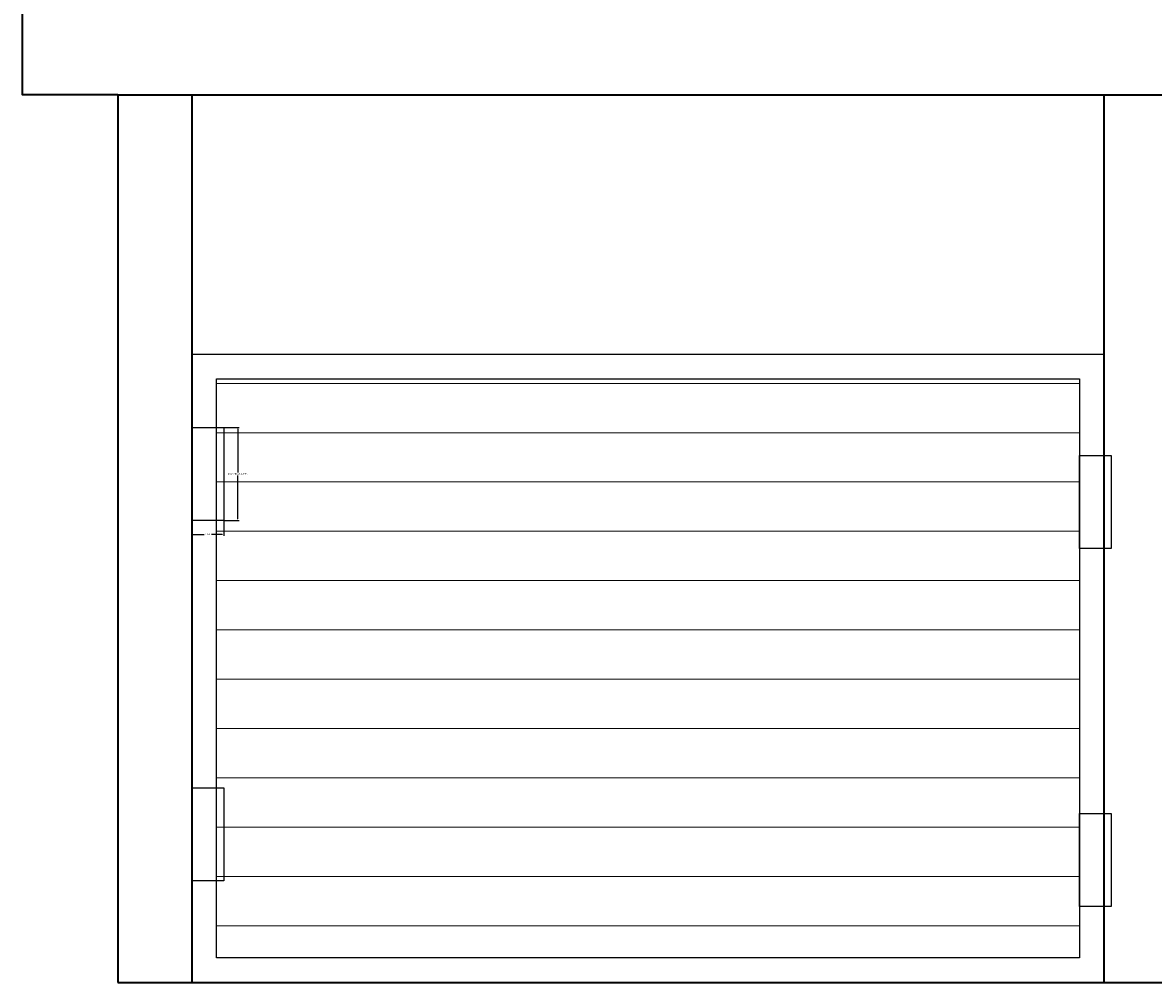
# Model space of a CAD drawing. Units: inches. Extents: x 3 to 303, y 4 to 326.
# Tile 1 of 6: x 4 to 141, y 4 to 120. Entities that reach past the tile are written whole.
import ezdxf

# ---------------------------------------------------------------- set-up
doc = ezdxf.new("R2010")
doc.units = ezdxf.units.IN
doc.header["$MEASUREMENT"] = 0
for name, color, linetype, lineweight in [('A-ANNO-DIMS', 2, 'Continuous', 18), ('A-DOOR', 3, 'Continuous', 25), ('A-ELEV', 7, 'Continuous', 35), ('A-ELEV-PATT', 8, 'Continuous', 13)]:
    doc.layers.add(name, color=color, linetype=linetype, lineweight=lineweight)
doc.styles.get("Standard").update_dxf_attribs({"font": 'arial.ttf'})
doc.dimstyles.get("Standard").update_dxf_attribs({"dimtxt": 0.18, "dimasz": 0.18, "dimexe": 0.18, "dimexo": 0.0625, "dimgap": 0.09, "dimtad": 0, "dimtih": 1, "dimtoh": 1, "dimdec": 4, "dimzin": 0, "dimdsep": 46, "dimtxsty": 'Standard', "dimcen": 0.09, "dimadec": 0, "dimazin": 0, "dimtfac": 1, "dimtdec": 4, "dimtofl": 0, "dimtmove": 0, "dimatfit": 3, "dimfxl": 1, "dimtolj": 1, "dimtzin": 0, "dimarcsym": 0})

# ---------------------------------------------------------------- blocks, each defined once
blk = doc.blocks.new('HINGE')
blk.add_lwpolyline([(171.8, 207.5), (175.68, 207.5), (175.68, 196.19), (171.8, 196.19)], close=True)
blk = doc.blocks.new('*D6')
at = {"layer": 'A-ANNO-DIMS', "color": 0, "lineweight": -2, "transparency": 16777216}
for p, q in [((28.18, 71.14), (29.99, 71.14)), ((29.81, 70.96), (29.81, 65.67)), ((29.81, 60.01), (29.81, 65.3)), ((28.18, 59.83), (29.99, 59.83))]:
    blk.add_line(p, q, dxfattribs=at)
at = {"layer": 'A-ANNO-DIMS', "color": 0, "transparency": 16777216}
for points in [[(29.78, 70.96), (29.84, 70.96), (29.81, 71.14)], [(29.78, 60.01), (29.84, 60.01), (29.81, 59.83)]]:
    blk.add_solid(points, dxfattribs=at)
at = {"layer": 'Defpoints', "color": 0, "transparency": 16777216}
for p in [(28.11, 71.14), (29.81, 71.14), (28.11, 59.83)]:
    blk.add_point(p, dxfattribs=at)
at = {"layer": 'A-ANNO-DIMS', "color": 0, "transparency": 16777216, "insert": (29.81, 65.49), "char_height": 0.18, "attachment_point": 5}
blk.add_mtext('\\A1;DOOR HINGE 11 TYP.', dxfattribs=at)
blk = doc.blocks.new('*D7')
at = {"layer": 'A-ANNO-DIMS', "color": 0, "lineweight": -2, "transparency": 16777216}
for p, q in [((24.23, 59.77), (24.23, 57.95)), ((28.11, 59.77), (28.11, 57.95)), ((24.41, 58.13), (25.71, 58.13)), ((27.93, 58.13), (26.63, 58.13))]:
    blk.add_line(p, q, dxfattribs=at)
at = {"layer": 'A-ANNO-DIMS', "color": 0, "transparency": 16777216}
for points in [[(24.41, 58.16), (24.41, 58.1), (24.23, 58.13)], [(27.93, 58.16), (27.93, 58.1), (28.11, 58.13)]]:
    blk.add_solid(points, dxfattribs=at)
at = {"layer": 'Defpoints', "color": 0, "transparency": 16777216}
for p in [(24.23, 59.83), (28.11, 59.83), (28.11, 58.13)]:
    blk.add_point(p, dxfattribs=at)
at = {"layer": 'A-ANNO-DIMS', "color": 0, "transparency": 16777216, "insert": (26.17, 58.13), "char_height": 0.18, "attachment_point": 5}
blk.add_mtext('\\A1;4 TYP.', dxfattribs=at)

msp = doc.modelspace()

# ---------------------------------------------------------------- hatches: boundary and pattern name
at = {"layer": 'A-ELEV-PATT'}
h = msp.add_hatch(dxfattribs=at)
h.set_pattern_fill('_USER', color=256, scale=6, pattern_type=0)
h.set_pattern_definition([(0, (-9.712, -25.502), (0, 6), [])])
h.paths.add_polyline_path([(132.23, 77.06), (27.23, 77.06), (27.23, 6.62), (132.23, 6.62)])

# ---------------------------------------------------------------- linework, layer by layer
at = {"layer": 'A-DOOR'}
for points in [[(24.23, 80.06), (135.23, 80.06), (135.23, 3.62), (24.23, 3.62)], [(27.23, 77.06), (132.23, 77.06), (132.23, 6.62), (27.23, 6.62)]]:
    msp.add_lwpolyline(points, close=True, dxfattribs=at)
at = {"layer": 'A-ELEV'}
for p, q in [((15.23, 111.62), (15.23, 3.62)), ((15.23, 111.62), (219.23, 111.62)), ((24.23, 111.62), (24.23, 3.62)), ((135.23, 3.62), (135.23, 111.62)), ((15.23, 3.62), (303.23, 3.62))]:
    msp.add_line(p, q, dxfattribs=at)
msp.add_lwpolyline([(15.23, 111.62), (3.64, 111.62), (3.64, 123.62), (15.23, 123.62)], dxfattribs=at)

# ---------------------------------------------------------------- block references
at = {"layer": 'A-DOOR'}
for p in [(-147.57, -136.36), (-39.57, -139.78), (-147.57, -180.22), (-39.57, -183.35)]:
    msp.add_blockref('HINGE', p, dxfattribs=at)

# ---------------------------------------------------------------- dimensions: what is measured, and where the dimension line sits
at = {"layer": 'A-ANNO-DIMS'}
dim = msp.add_linear_dim(base=(29.81, 71.14), p1=(28.11, 59.83), p2=(28.11, 71.14), angle=90, text='DOOR HINGE <> TYP.', dimstyle='Standard', override={"dimdec": 0, "dimlfac": 1, "dimrnd": 0, "dimzin": 0, "dimdsep": 46, "dimlunit": 2}, dxfattribs=at)
dim.commit()
dim.dimension.update_dxf_attribs({"geometry": '*D6', "text_midpoint": (29.81, 65.49)})
dim = msp.add_linear_dim(base=(28.11, 58.13), p1=(24.23, 59.83), p2=(28.11, 59.83), text='<> TYP.', dimstyle='Standard', override={"dimdec": 0, "dimlfac": 1, "dimrnd": 0, "dimzin": 0, "dimdsep": 46, "dimlunit": 2}, dxfattribs=at)
dim.commit()
dim.dimension.update_dxf_attribs({"geometry": '*D7', "text_midpoint": (26.17, 58.13)})

doc.saveas('drawing.dxf')
